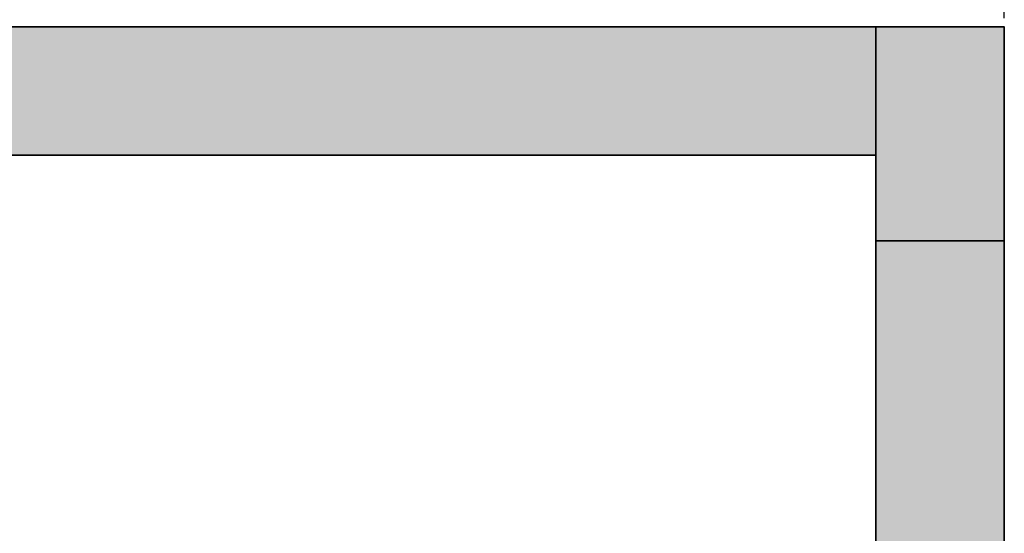
# Model space of a CAD drawing. Units: inches. Extents: x 3148 to 3962, y 1142 to 1671.
# Tile 5 of 9: x 3413 to 3482, y 1519 to 1555. Entities that reach past the tile are written whole.
import ezdxf

# ---------------------------------------------------------------- set-up
doc = ezdxf.new("R2010")
doc.units = ezdxf.units.IN
for name, color, linetype, lineweight in [('A-ANNO-DIMS', 2, 'Continuous', 18), ('A-COLS', 1, 'Continuous', 35), ('A-WALL', 7, 'Continuous', 35)]:
    doc.layers.add(name, color=color, linetype=linetype, lineweight=lineweight)
doc.layers.add('A-WALL-PATT', color=252, linetype='Continuous', lineweight=13, true_color=0x939598)
doc.styles.get("Standard").update_dxf_attribs({"font": 'arial.ttf'})
doc.dimstyles.new('ISO-25', dxfattribs={"dimtxt": 9, "dimasz": 2.5, "dimexe": 1.25, "dimexo": 0.625, "dimtad": 1, "dimdec": 1, "dimlunit": 3, "dimtxsty": 'Standard', "dimcen": 2.5, "dimadec": 0, "dimazin": 0, "dimtfac": 1, "dimtdec": 1, "dimtmove": 0, "dimatfit": 3, "dimfxl": 1, "dimarcsym": 0})

# ---------------------------------------------------------------- blocks, each defined once
blk = doc.blocks.new('*D42')
at = {"layer": 'A-ANNO-DIMS', "color": 0, "lineweight": -2, "transparency": 16777216}
for p, q in [((3194.042306275787, 1555.424200034517), (3194.042306275787, 1571.690472151851)), ((3482.042306275788, 1555.424200034517), (3482.042306275788, 1571.690472151851)), ((3196.542306275788, 1570.440472151851), (3479.542306275788, 1570.440472151851))]:
    blk.add_line(p, q, dxfattribs=at)
at = {"layer": 'A-ANNO-DIMS', "color": 0, "transparency": 16777216}
for points in [[(3196.542306275788, 1570.857138818518), (3196.542306275788, 1570.023805485184), (3194.042306275787, 1570.440472151851)], [(3479.542306275788, 1570.857138818518), (3479.542306275788, 1570.023805485184), (3482.042306275788, 1570.440472151851)]]:
    blk.add_solid(points, dxfattribs=at)
at = {"layer": 'Defpoints', "color": 0, "transparency": 16777216}
for p in [(3482.042306275788, 1570.440472151851), (3194.042306275787, 1554.799200034517), (3482.042306275788, 1554.799200034517)]:
    blk.add_point(p, dxfattribs=at)
at = {"layer": 'A-ANNO-DIMS', "color": 0, "transparency": 16777216, "insert": (3338.042306275787, 1575.583889614334), "char_height": 9, "attachment_point": 5}
blk.add_mtext("24'", dxfattribs=at)
blk = doc.blocks.new('COL-9X15')
h = blk.add_hatch(color=256)
h.dxf.hatch_style = 1
h.paths.add_polyline_path([(9.000306275787352, 15.00020003451709), (0.0003062757873522, 15.00020003451709), (0.0003062757873522, 0.0002000345170927), (9.000306275787352, 0.0002000345170927)])
blk.add_lwpolyline([(9.000306275787352, 0.0002000345170927), (9.000306275787352, 15.00020003451709), (0.0003062757873522, 15.00020003451709), (0.0003062757873522, 0.0002000345170927)], close=True)

msp = doc.modelspace()

# ---------------------------------------------------------------- hatches: boundary and pattern name
at = {"layer": 'A-WALL-PATT'}
h = msp.add_hatch(color=256, dxfattribs=at)
h.dxf.hatch_style = 1
h.paths.add_polyline_path([(3203.042306275788, 1410.799200034518), (3194.042306275787, 1410.799200034518), (3194.042306275787, 1296.799200034517), (3203.042306275786, 1296.799200034517), (3203.042306275787, 1300.855382799943)])
h.paths.add_polyline_path([(3203.042306275778, 1281.799200034517), (3194.042306275787, 1281.799200034517), (3194.042306275787, 1212.799200034517), (3203.042306275788, 1212.799200034517)])
h.paths.add_polyline_path([(3326.042306275788, 1206.799200034517), (3203.042306275788, 1206.799200034517), (3203.042306275788, 1197.799200034517), (3326.042306275788, 1197.799200034517)])
h.paths.add_polyline_path([(3341.042306275787, 1362.799200034517), (3335.042306275788, 1362.799200034517), (3335.042306275788, 1290.799200034517), (3341.042306275787, 1290.799200034517)])
h.paths.add_polyline_path([(3341.042306275788, 1207.799200034517), (3335.042306275788, 1207.799200034517), (3335.042306275788, 1206.799200034517), (3341.042306275788, 1206.799200034517)])
h.paths.add_polyline_path([(3341.042306275787, 1259.799200034517), (3335.042306275788, 1259.799200034517), (3335.042306275788, 1255.799200034517), (3341.042306275787, 1255.799200034517)])
h.paths.add_polyline_path([(3341.042306275787, 1281.799200034517), (3335.042306275788, 1281.799200034517), (3335.042306275788, 1277.799200034517), (3341.042306275787, 1277.799200034517)])
h.paths.add_polyline_path([(3377.042306275787, 1287.799200034517), (3350.042306275788, 1287.799200034517), (3350.042306275788, 1281.799200034517), (3377.042306275787, 1281.799200034517)])
h.paths.add_polyline_path([(3473.042306275787, 1287.799200034517), (3445.042307275787, 1287.799200034517), (3437.042306275787, 1287.799200034517), (3437.042306275788, 1281.799200034517), (3473.042306275787, 1281.799200034517)])
h.paths.add_polyline_path([(3482.042306275788, 1313.299200034517), (3473.042306275787, 1313.299200034517), (3473.042306275787, 1296.799200034517), (3482.042306275788, 1296.799200034517)])
h.paths.add_polyline_path([(3482.042306275788, 1410.799200034517), (3473.042306275787, 1410.799200034517), (3473.042306275787, 1385.299200034517), (3482.042306275788, 1385.299200034517)])
h.paths.add_polyline_path([(3473.042306275787, 1416.799200034517), (3344.042306275788, 1416.799200034517), (3344.042306275788, 1410.799200034517), (3473.042306275787, 1410.799200034517)])
h.paths.add_polyline_path([(3482.042306275788, 1445.299200034517), (3473.042306275787, 1445.299200034517), (3473.042306275787, 1425.799200034517), (3482.042306275788, 1425.799200034517)])
h.paths.add_polyline_path([(3341.042306275787, 1426.299200034517), (3335.042306275788, 1426.299200034517), (3335.042306275788, 1425.799200034517), (3341.042306275787, 1425.799200034517)])
h.paths.add_polyline_path([(3304.042306275788, 1428.799200034517), (3253.542306275787, 1428.799200034517), (3253.542306275788, 1430.299200034517), (3251.042306275788, 1430.299200034517), (3251.042306275787, 1428.799200034517), (3203.042306275788, 1428.799200034517), (3203.042306275788, 1512.799200034517), (3215.042306275788, 1512.799200034517), (3215.042306275788, 1518.799200034517), (3203.042306275788, 1518.799200034517), (3203.042306275788, 1539.799200034517), (3194.042306275787, 1539.799200034517), (3194.042306275787, 1425.799200034519), (3203.042306275787, 1425.799200034519), (3203.042306275787, 1422.799200034517), (3304.042306275788, 1422.799200034517)])
h.paths.add_polyline_path([(3265.542306275789, 1518.799200034517), (3239.042306275788, 1518.799200034517), (3239.042306275788, 1512.799200034517), (3251.042306275788, 1512.799200034517), (3251.042306275788, 1461.299200034517), (3253.542306275789, 1461.299200034517), (3253.542306275789, 1462.299200034517), (3255.542306275788, 1462.299200034517), (3255.542306275788, 1464.799200034517), (3253.542306275789, 1464.799200034517), (3253.542306275788, 1512.799200034517), (3265.542306275789, 1512.799200034517)], flags=17)
h.paths.add_polyline_path([(3307.542306275788, 1518.799200034517), (3289.542306275789, 1518.799200034517), (3289.542306275789, 1512.799200034517), (3301.542306275788, 1512.799200034517), (3301.542306275788, 1464.799200034517), (3286.542306275788, 1464.799200034517), (3286.542306275788, 1462.299200034517), (3304.042306275788, 1462.299200034517), (3304.042306275788, 1512.799200034517), (3307.542306275788, 1512.799200034517)])
h.paths.add_polyline_path([(3341.042306275787, 1539.799200034517), (3335.042306275788, 1539.799200034517), (3335.042306275788, 1518.799200034517), (3331.542306275788, 1518.799200034517), (3331.542306275788, 1512.799200034517), (3335.042306275788, 1512.799200034517), (3335.042306275788, 1462.299200034517), (3341.042306275787, 1462.299200034517)])
h.paths.add_polyline_path([(3335.042306275788, 1554.799200034517), (3203.042306275788, 1554.799200034517), (3203.042306275788, 1545.799200034517), (3335.042306275788, 1545.799200034517)])
h.paths.add_polyline_path([(3473.042306275787, 1554.799200034517), (3344.042306275787, 1554.799200034517), (3344.042306275787, 1545.799200034517), (3362.939954275788, 1545.799200034517), (3473.042306275787, 1545.799200034517)])
h.paths.add_polyline_path([(3482.042306275788, 1539.799200034517), (3473.042306275787, 1539.799200034517), (3473.042306275787, 1517.299200034517), (3482.042306275788, 1517.299200034517)])

# ---------------------------------------------------------------- linework, layer by layer
at = {"layer": 'A-WALL'}
for p, q in [((3194.042306275787, 1554.799200034517), (3482.042306275788, 1554.799200034517)), ((3482.042306275788, 1554.799200034517), (3482.042306275788, 1281.799200034517)), ((3341.042306275787, 1545.799200034517), (3473.042306275787, 1545.799200034517)), ((3473.042306275787, 1545.799200034517), (3473.042306275787, 1416.799200034517))]:
    msp.add_line(p, q, dxfattribs=at)

# ---------------------------------------------------------------- block references
at = {"layer": 'A-COLS'}
msp.add_blockref('COL-9X15', (3473.042000000001, 1539.799), dxfattribs=at)

# ---------------------------------------------------------------- dimensions: what is measured, and where the dimension line sits
at = {"layer": 'A-ANNO-DIMS'}
dim = msp.add_linear_dim(base=(3482.042306275788, 1570.440472151851), p1=(3194.042306275787, 1554.799200034517), p2=(3482.042306275788, 1554.799200034517), dimstyle='ISO-25', override={"dimclrd": 0, "dimclre": 0, "dimclrt": 0}, dxfattribs=at)
dim.commit()
dim.dimension.update_dxf_attribs({"geometry": '*D42', "text_midpoint": (3338.042306275787, 1575.583889614334)})

doc.saveas('drawing.dxf')
